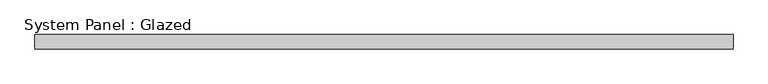
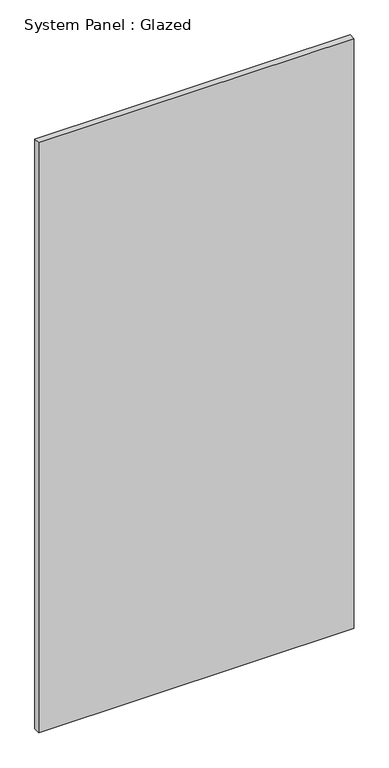
"""IFC4 building model written with IfcOpenShell, lengths in millimetres: plate geometry, System Panel : Glazed."""

from ifc_helpers import new_model, si_unit, origin, origin_with_axes, place, context, project, spatial, polyline, outline, extrude, source, transform, mapped, element, save


def system_panel_glazed_7ffa2d15(model_context):
    return source(origin(), model_context, "Body", "SweptSolid", [
        extrude(outline(polyline([(622.3, 19.05), (-622.3, 19.05), (-622.3, 44.45), (622.3, 44.45), (622.3, 19.05)])), origin_with_axes(), (0.0, 0.0, 1.0), 2463.8),
    ])


if __name__ == "__main__":
    model = new_model("IFC4")
    model_context = context("Model", 3, world=origin())
    ifc_project = project(units=[si_unit("LENGTHUNIT", "METRE", prefix="MILLI")], contexts=[model_context])
    site = spatial("IfcSite", under=ifc_project)
    building = spatial("IfcBuilding", under=site)
    placement = place(None, origin())
    system_panel_glazed_shape = system_panel_glazed_7ffa2d15(model_context)
    element("IfcPlate", 1, ObjectType="System Panel : Glazed", at=placement, inside=building, context=model_context, shape_type="MappedRepresentation", body=[
        mapped(system_panel_glazed_shape, transform((0.0, 0.0, 0.0), x_axis=(1.0, 0.0, 0.0), y_axis=(0.0, 1.0, 0.0), z_axis=(0.0, 0.0, 1.0))),
    ])
    save(model, "model.ifc")

# Revit data of these elements
# Type "System Panel : Glazed"
#   Construction Type Id = "GSP4R"
#   Analytic Construction = "1/8 in Pilkington single glazing"
#   Visual Light Transmittance = 0.9
#   Solar Heat Gain Coefficient = 0.86
#   Heat Transfer Coefficient (U) = 1.18115 BTU/(h·ft²·°F)
#   Define Thermal Properties by = 1
# Element 1 (IfcPlate, "System Panel : Glazed")
#   Materials on its faces: "Glass"
# Materials
#   "Glass": class "Glass", colour RGB 0 128 192, transparency 0.75, Description = "Soda Lime Glass", Cost = 0
